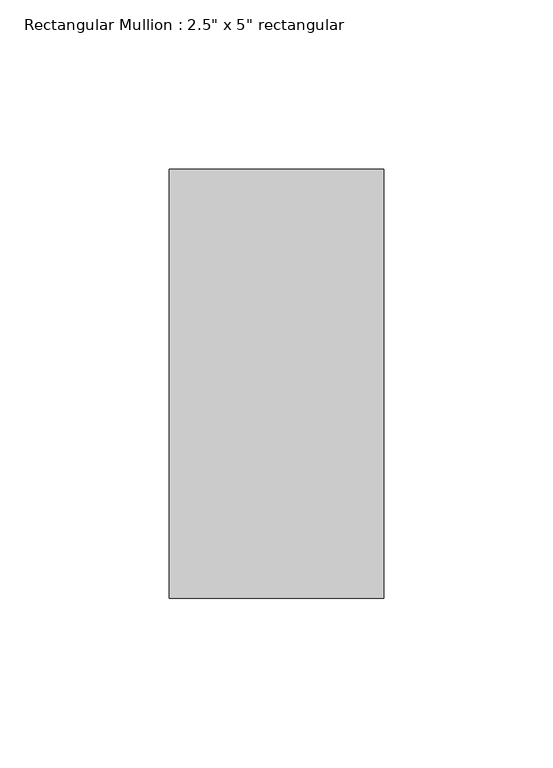
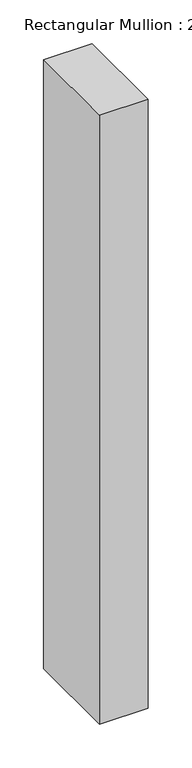
"""IFC4 building model written with IfcOpenShell, lengths in millimetres: member geometry."""

from ifc_helpers import new_model, si_unit, frame, origin, place, context, project, spatial, polyline, outline, extrude, source, transform, mapped, element, save


def member_091e92f8(model_context):
    return source(origin(), model_context, "Body", "SweptSolid", [
        extrude(outline(polyline([(0.0, 63.5), (0.0, -63.5), (-63.5, -63.5), (-63.5, 63.5), (0.0, 63.5)])), frame((0.0, 0.0, -844.55), z_axis=(0.0, 0.0, 1.0), x_axis=(1.0, 0.0, 0.0)), (0.0, 0.0, 1.0), 844.55),
    ])


if __name__ == "__main__":
    model = new_model("IFC4")
    model_context = context("Model", 3, world=origin())
    ifc_project = project(units=[si_unit("LENGTHUNIT", "METRE", prefix="MILLI")], contexts=[model_context])
    site = spatial("IfcSite", under=ifc_project)
    building = spatial("IfcBuilding", under=site)
    placement = place(None, origin())
    member_shape = member_091e92f8(model_context)
    element("IfcMember", 1, ObjectType="Rectangular Mullion : 2.5\" x 5\" rectangular", at=placement, inside=building, context=model_context, shape_type="MappedRepresentation", body=[
        mapped(member_shape, transform((0.0, 0.0, 0.0), x_axis=(1.0, 0.0, 0.0), y_axis=(0.0, 1.0, 0.0), z_axis=(0.0, 0.0, 1.0))),
    ])
    save(model, "model.ifc")

# Revit data of these elements
# Type "Rectangular Mullion : 2.5\" x 5\" rectangular"
#   built-in parameter 1007304 = 0.416667 (stored number, unit not read)
#   built-in parameter 1007301 = 0.104167 (stored number, unit not read)
#   built-in parameter 1007300 = 0.104167 (stored number, unit not read)
